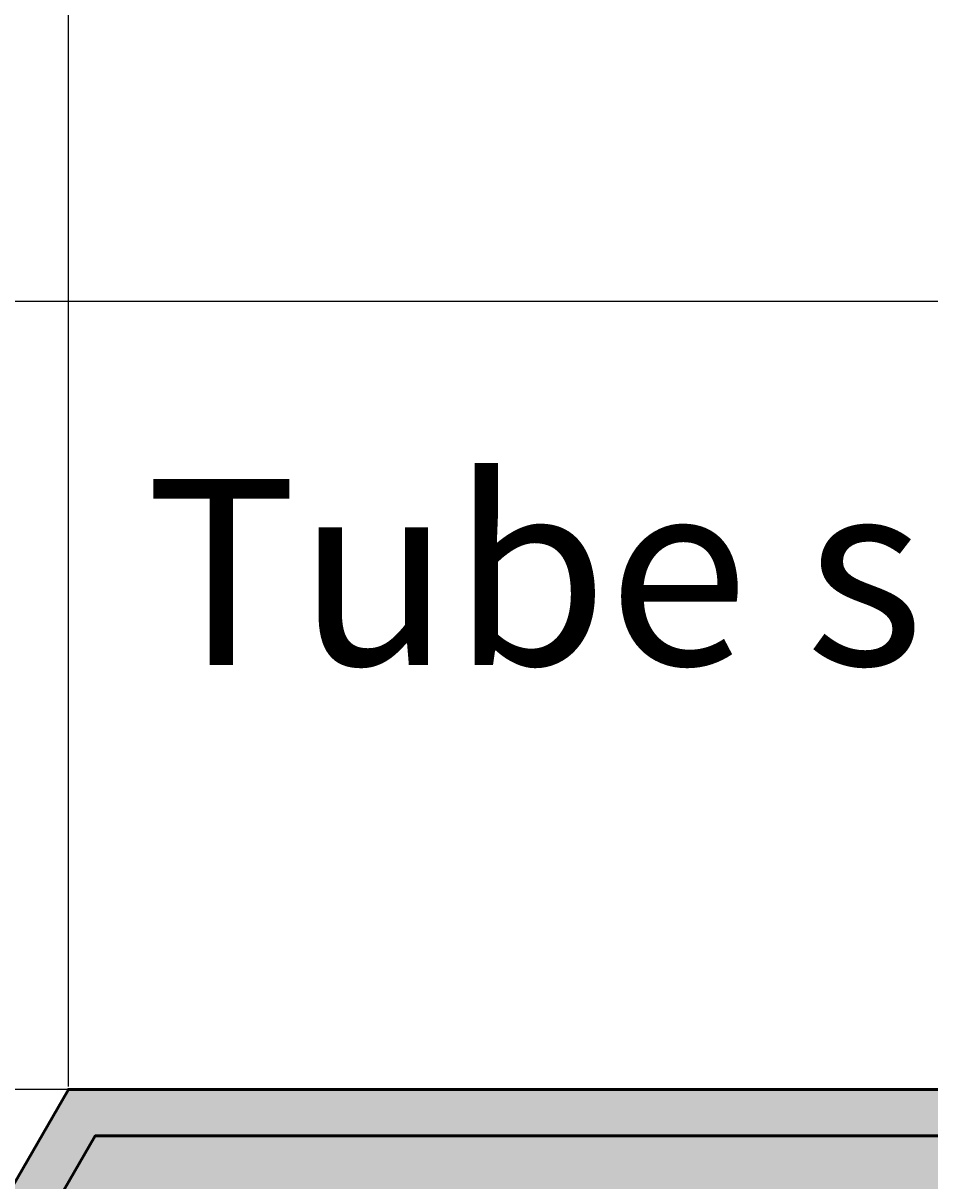
# Model space of a CAD drawing. Units: inches. Extents: x -12 to 334, y -10 to 186.
# Tile 60 of 77: x 125 to 145, y 136 to 161. Entities that reach past the tile are written whole.
import ezdxf
from ezdxf import colors
from ezdxf.entities.mleader import LeaderData, LeaderLine
from ezdxf.math import Vec2, Vec3

# ---------------------------------------------------------------- set-up
doc = ezdxf.new("R2010")
doc.units = ezdxf.units.IN
doc.header["$MEASUREMENT"] = 0
for name, color, linetype, lineweight in [('M-ANNO-TEXT', 3, 'Continuous', 25), ('M-DIMS', 2, 'Continuous', 18), ('M-EQPM', 7, 'Continuous', 50), ('M-EQPM-PATT', 8, 'Continuous', 18)]:
    doc.layers.add(name, color=color, linetype=linetype, lineweight=lineweight)
doc.styles.get("Standard").update_dxf_attribs({"font": 'arial.ttf'})
doc.dimstyles.get("Standard").update_dxf_attribs({"dimtxt": 0.18, "dimasz": 0.18, "dimexe": 0.18, "dimexo": 0.0625, "dimgap": 0.09, "dimtad": 0, "dimtih": 1, "dimtoh": 1, "dimdec": 4, "dimzin": 0, "dimdsep": 46, "dimtxsty": 'Standard', "dimcen": 0.09, "dimadec": 0, "dimazin": 0, "dimtfac": 1, "dimtdec": 4, "dimtofl": 0, "dimtmove": 0, "dimatfit": 3, "dimfxl": 1, "dimtolj": 1, "dimtzin": 0, "dimarcsym": 0})

# ---------------------------------------------------------------- blocks, each defined once
blk = doc.blocks.new('*D16')
at = {"layer": 'Defpoints', "color": 0, "transparency": 16777216}
for p in [(126.379, 169.385), (126.379, 137.887), (106.177, 102.896)]:
    blk.add_point(p, dxfattribs=at)
at = {"layer": 'M-DIMS', "color": 0, "lineweight": -2, "transparency": 16777216}
for p, q in [((106.177, 102.958), (106.177, 169.565)), ((106.357, 169.385), (115.814, 169.385)), ((126.199, 169.385), (116.742, 169.385)), ((126.379, 137.95), (126.379, 169.565))]:
    blk.add_line(p, q, dxfattribs=at)
at = {"layer": 'M-DIMS', "color": 0, "transparency": 16777216}
for points in [[(106.357, 169.415), (106.357, 169.355), (106.177, 169.385)], [(126.199, 169.415), (126.199, 169.355), (126.379, 169.385)]]:
    blk.add_solid(points, dxfattribs=at)
at = {"layer": 'M-DIMS', "color": 0, "transparency": 16777216, "insert": (116.278, 169.385), "char_height": 0.18, "attachment_point": 5}
blk.add_mtext('\\A1;20.202', dxfattribs=at)
blk = doc.blocks.new('*D18')
at = {"layer": 'Defpoints', "color": 0, "transparency": 16777216}
for p in [(190.342, 169.385), (190.342, 154.835), (126.379, 137.887)]:
    blk.add_point(p, dxfattribs=at)
at = {"layer": 'M-DIMS', "color": 0, "lineweight": -2, "transparency": 16777216}
for p, q in [((126.379, 137.95), (126.379, 169.565)), ((126.559, 169.385), (157.967, 169.385)), ((190.162, 169.385), (158.755, 169.385)), ((190.342, 154.897), (190.342, 169.565))]:
    blk.add_line(p, q, dxfattribs=at)
at = {"layer": 'M-DIMS', "color": 0, "transparency": 16777216}
for points in [[(126.559, 169.415), (126.559, 169.355), (126.379, 169.385)], [(190.162, 169.415), (190.162, 169.355), (190.342, 169.385)]]:
    blk.add_solid(points, dxfattribs=at)
at = {"layer": 'M-DIMS', "color": 0, "transparency": 16777216, "insert": (158.361, 169.385), "char_height": 0.18, "attachment_point": 5}
blk.add_mtext('\\A1;63.96', dxfattribs=at)
blk = doc.blocks.new('*D22')
at = {"layer": 'Defpoints', "color": 0, "transparency": 16777216}
for p in [(190.342, 154.835), (-11.174, 137.887), (195.342, 137.887)]:
    blk.add_point(p, dxfattribs=at)
at = {"layer": 'M-DIMS', "color": 0, "lineweight": -2, "transparency": 16777216}
for p, q in [((190.28, 154.835), (-11.354, 154.835)), ((-11.174, 154.655), (-11.174, 146.543)), ((-11.174, 138.067), (-11.174, 146.179)), ((195.28, 137.887), (-11.354, 137.887))]:
    blk.add_line(p, q, dxfattribs=at)
at = {"layer": 'M-DIMS', "color": 0, "transparency": 16777216}
for points in [[(-11.204, 154.655), (-11.144, 154.655), (-11.174, 154.835)], [(-11.204, 138.067), (-11.144, 138.067), (-11.174, 137.887)]]:
    blk.add_solid(points, dxfattribs=at)
at = {"layer": 'M-DIMS', "color": 0, "transparency": 16777216, "insert": (-11.174, 146.361), "char_height": 0.18, "attachment_point": 5}
blk.add_mtext('\\A1;16.947', dxfattribs=at)

msp = doc.modelspace()

# ---------------------------------------------------------------- hatches: boundary and pattern name
at = {"layer": 'M-EQPM-PATT', "transparency": 33554556}
h = msp.add_hatch(color=256, dxfattribs=at)
h.set_gradient(color1=(248, 206, 179), color2=(248, 206, 179), tint=1)
h.paths.add_polyline_path([(179.7818, 136.8871), (126.9567, 136.8871), (106.1771, 100.8958), (171.5458, 100.8958)])
h.paths.add_polyline_path([(268.3808, 136.9435), (214.0166, 136.9435), (214.0166, 154.8345), (196.3421, 154.8345), (196.3421, 136.8871), (179.7818, 136.8871), (171.5458, 100.8958), (231.7758, 100.8958, -0.4142136), (251.9801, 80.6915), (279.7263, 80.6915, 0.1631825)])
at = {"layer": 'M-EQPM-PATT'}
h = msp.add_hatch(color=256, dxfattribs=at)
h.set_gradient(color1=(99, 100, 102), color2=(99, 100, 102), tint=1)
h.paths.add_polyline_path([(126.9567, 136.8871), (179.7818, 136.8871), (180.0106, 137.8871), (126.3793, 137.8871), (106.1771, 102.8958), (86.8879, 102.8958), (86.8879, 109.0583), (84.7229, 109.0583), (84.7229, 100.8958), (106.1771, 100.8958)])
h.paths.add_polyline_path([(196.3421, 152.8345), (195.3421, 152.8345), (195.3421, 137.8871), (180.0106, 137.8871), (179.7818, 136.8871), (196.3421, 136.8871)])
h.paths.add_polyline_path([(215.0166, 152.8345), (214.0166, 152.8345), (214.0166, 136.9435), (268.3808, 136.9435, -0.2673785), (268.3808, 46.8541), (249.3759, 46.8541), (249.8485, 45.8541), (269.3808, 45.8541, 0.2615891), (269.3808, 137.9435), (215.0166, 137.9435)])

# ---------------------------------------------------------------- linework, layer by layer
at = {"layer": 'M-EQPM'}
for points in [[(106.1771, 100.8958), (126.9567, 136.8871), (196.3421, 136.8871), (196.3421, 154.8345)], [(106.1771, 102.8958), (126.3793, 137.8871), (195.3421, 137.8871), (195.3421, 152.8345)]]:
    msp.add_lwpolyline(points, dxfattribs=at)

# ---------------------------------------------------------------- dimensions: what is measured, and where the dimension line sits
at = {"layer": 'M-DIMS'}
for base, p1, p2, override, picture, middle in [((126.3793, 169.3845), (106.1771, 102.8958), (126.3793, 137.8871), {"dimdec": 3, "dimlfac": 1, "dimrnd": 0, "dimzin": 0, "dimdsep": 46, "dimlunit": 2}, '*D16', (116.2782, 169.3845)), ((190.3421, 169.3845), (126.3793, 137.8871), (190.3421, 154.8345), {"dimdec": 2, "dimlfac": 1, "dimrnd": 0, "dimzin": 0, "dimdsep": 46, "dimlunit": 2}, '*D18', (158.3607, 169.3845))]:
    dim = msp.add_linear_dim(base=base, p1=p1, p2=p2, dimstyle='Standard', override=override, dxfattribs=at)
    dim.commit()
    dim.dimension.update_dxf_attribs({"geometry": picture, "text_midpoint": middle})
dim = msp.add_linear_dim(base=(-11.1736, 137.8871), p1=(190.3421, 154.8345), p2=(195.3421, 137.8871), angle=90, dimstyle='Standard', override={"dimdec": 3, "dimlfac": 1, "dimrnd": 0, "dimzin": 0, "dimdsep": 46, "dimlunit": 2}, dxfattribs=at)
dim.commit()
dim.dimension.update_dxf_attribs({"geometry": '*D22', "text_midpoint": (-11.1735, 146.3608)})

# ---------------------------------------------------------------- leaders
at = {"layer": 'M-ANNO-TEXT'}
ml = msp.add_multileader_mtext('Standard', dxfattribs=at)
ml.set_content('Tube supports', color=256)
ml.set_leader_properties()
ml.build(insert=Vec2(0, 0))
ml.multileader.update_dxf_attribs({"dogleg_length": 0.36, "arrow_head_size": 0.7})
ctx = ml.context
ctx.base_point, ctx.arrow_head_size, ctx.landing_gap_size, ctx.plane_origin = Vec3(129.4363, 148.4609), 0.7, 0.09, Vec3(117.375, 151.6517)
ctx.text_align_type = 2
notes = []
notes.append((ctx, [(1, (1, 1, 0), (182.4302, 148.4609), (-1, 0), 17.4388, [(0, [(170.9079, 98.1081)], 0, [])])]))
ctx.mtext.insert, ctx.mtext.alignment, ctx.mtext.flow_direction = Vec3(164.9015, 151.0162), 3, 5
for ctx, leaders in notes:
    for number, flags, end, landing, length, lines in leaders:
        leader = LeaderData()
        leader.index, (leader.has_last_leader_line, leader.has_dogleg_vector, leader.attachment_direction) = number, flags
        leader.last_leader_point, leader.dogleg_vector, leader.dogleg_length = Vec3(end), Vec3(landing), length
        for number, points, colour, breaks in lines:
            line = LeaderLine()
            line.index, line.vertices, line.color, line.breaks = number, Vec3.list(points), colors.encode_raw_color(colour), breaks
            leader.lines.append(line)
        ctx.leaders.append(leader)

doc.saveas('drawing.dxf')
